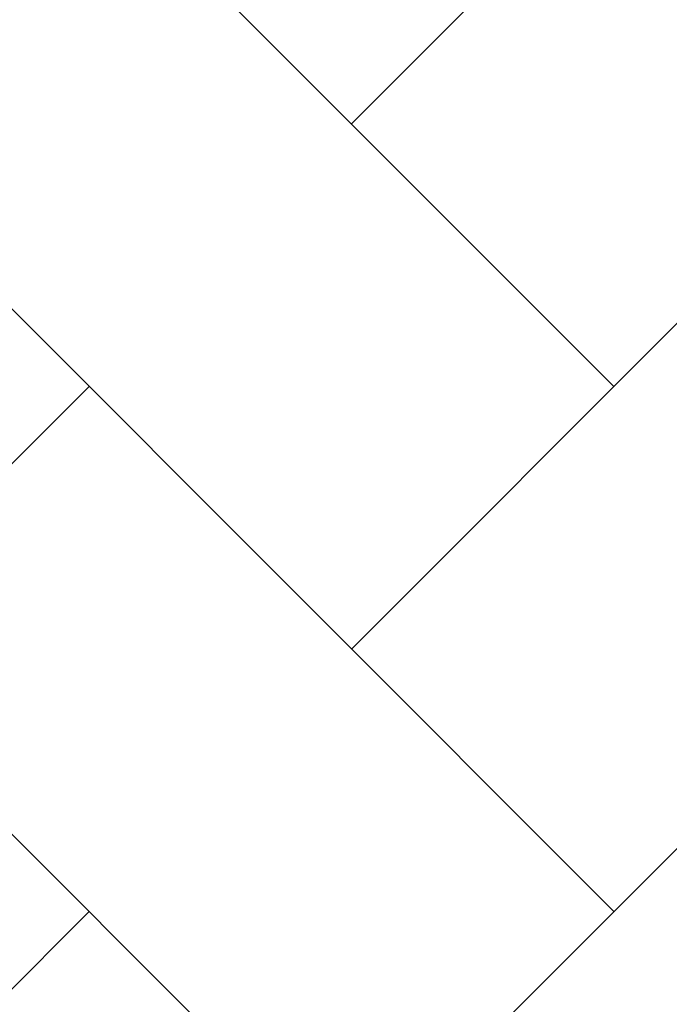
# Model space of a CAD drawing. Units: inches. Extents: x 3590 to 5167, y 65 to 1917.
# Tile 55 of 100: x 4968 to 5003, y 1504 to 1558. Entities that reach past the tile are written whole.
import ezdxf

# ---------------------------------------------------------------- set-up
doc = ezdxf.new("R2010")
doc.units = ezdxf.units.IN
doc.layers.add('A-FLOR-PATT', color=8, linetype='Continuous', lineweight=13)

msp = doc.modelspace()

# ---------------------------------------------------------------- hatches: boundary and pattern name
at = {"layer": 'A-FLOR-PATT', "transparency": 33554687}
h = msp.add_hatch(dxfattribs=at)
h.set_pattern_fill('AR-HBONE', color=256, scale=0.2)
h.set_pattern_definition([(45, (-588.972, 0), (0, 28.73682), [60.96, -20.32]), (135, (-574.604, 14.368), (3e-15, 28.73682), [60.96, -20.32])])
h.paths.add_polyline_path([(5071.274, 1796.999), (4933.274, 1796.999), (4933.274, 1753.999), (4962.774, 1753.999, -0.414214), (4928.774, 1719.999), (4933.274, 1718.999), (4933.274, 1334.999), (5071.274, 1334.999)])
h.paths.add_polyline_path([(4951.78, 1521.077), (4951.715, 1521.04), (4951.563, 1520.895)], flags=16)
h.paths.add_polyline_path([(4952.267, 1521.376), (4952.198, 1521.371), (4952.198, 1521.356)], flags=0)
h.paths.add_polyline_path([(4967.051, 1529.728), (4965.231, 1528.694), (4963.411, 1527.714), (4961.756, 1526.851), (4963.589, 1527.449), (4964.036, 1527.478), (4962.975, 1527.249), (4961.76, 1526.852), (4959.792, 1525.834), (4958.005, 1524.895), (4956.24, 1523.93), (4954.504, 1522.919), (4954.129, 1522.682), (4953.361, 1521.997), (4953.366, 1521.998), (4953.605, 1522.064), (4955.106, 1522.761), (4956.921, 1523.434), (4958.678, 1523.915), (4960.358, 1524.2), (4961.945, 1524.286), (4964.171, 1524.108), (4965.958, 1523.309), (4963.863, 1522.976), (4965.187, 1522.499), (4963.366, 1522.497), (4961.545, 1522.487), (4959.764, 1522.461), (4958.304, 1522.419), (4957.974, 1522.388), (4956.307, 1522.232), (4954.718, 1522.071), (4953.251, 1521.899), (4953.525, 1521.623), (4954.331, 1521.379), (4956.243, 1521.23), (4958.039, 1520.93), (4959.684, 1520.483), (4961.16, 1519.896), (4963.107, 1518.8), (4964.393, 1517.325), (4962.973, 1517.726), (4964.558, 1516.661), (4965.407, 1515.708), (4963.507, 1516.322), (4961.68, 1517.005), (4959.935, 1517.745), (4958.282, 1518.528), (4956.732, 1519.343), (4955.295, 1520.175), (4954.672, 1520.572), (4954.513, 1520.627), (4955.658, 1519.318), (4956.703, 1517.982), (4957.644, 1516.647), (4958.485, 1515.334), (4959.55, 1513.524), (4960.438, 1511.769), (4958.841, 1513.62), (4957.452, 1515.325), (4955.819, 1517.459), (4956.665, 1515.448), (4957.111, 1513.923), (4957.447, 1511.714), (4957.076, 1509.793), (4956.538, 1511.11), (4955.992, 1512.569), (4955.444, 1514.125), (4954.898, 1515.735), (4954.357, 1517.356), (4953.824, 1518.943), (4953.305, 1520.452), (4953.065, 1521.116), (4952.971, 1521.146), (4952.949, 1521.086), (4952.73, 1520.199), (4953.37, 1518.024), (4953.757, 1516.373), (4954.051, 1514.765), (4954.264, 1513.221), (4954.471, 1511.131), (4954.497, 1510.402), (4954.409, 1511.76), (4954.264, 1513.221), (4954.051, 1514.765), (4953.757, 1516.373), (4953.37, 1518.024), (4952.877, 1519.698), (4952.716, 1520.141), (4952.533, 1519.059), (4952.374, 1517.789), (4952.219, 1516.312), (4952.046, 1514.6), (4951.833, 1512.626), (4951.557, 1510.363), (4951.203, 1512.168), (4950.852, 1514.339), (4950.985, 1516.376), (4951.66, 1518.286), (4952.593, 1520.481), (4952.357, 1521.13), (4951.855, 1520.328), (4950.839, 1518.908), (4949.777, 1517.587), (4948.916, 1516.617), (4948.111, 1515.256), (4947.089, 1513.554), (4945.889, 1511.615), (4946.326, 1513.402), (4946.562, 1514.249), (4945.528, 1513.327), (4944.581, 1512.531), (4946.018, 1514.508), (4947.204, 1516.048), (4947.893, 1517.313), (4949.307, 1518.764), (4950.414, 1519.767), (4950.451, 1519.806), (4952.267, 1521.376), (4951.645, 1521.493), (4950.404, 1521.18), (4948.044, 1520.359), (4946.119, 1519.452), (4944.572, 1518.475), (4943.35, 1517.443), (4941.997, 1515.92), (4941.661, 1515.275), (4942.813, 1516.99), (4944.572, 1518.475), (4946.119, 1519.452), (4948.044, 1520.359), (4950.404, 1521.18), (4951.645, 1521.493), (4949.647, 1521.868), (4948.6, 1521.756), (4947.126, 1521.57), (4945.42, 1521.348), (4943.45, 1521.105), (4941.183, 1520.856), (4942.86, 1521.613), (4943.873, 1522.03), (4942.952, 1521.909), (4941.41, 1521.485), (4939.543, 1520.67), (4938.968, 1520.226), (4940.733, 1521.299), (4942.952, 1521.909), (4943.702, 1522.008), (4945.894, 1522.7), (4947.565, 1522.714), (4948.921, 1522.566), (4951.131, 1522.183), (4950.971, 1522.297), (4948.129, 1523.006), (4946.035, 1523.707), (4944.232, 1524.521), (4942.707, 1525.461), (4941.444, 1526.537), (4940.43, 1527.761), (4939.649, 1529.143), (4941.421, 1528.122), (4943.147, 1527.132), (4944.841, 1526.175), (4946.514, 1525.25), (4948.179, 1524.359), (4948.365, 1524.263), (4946.475, 1526.045), (4945.181, 1527.54), (4944.19, 1529.033), (4943.496, 1530.54), (4943.278, 1531.36), (4942.498, 1531.919), (4943.114, 1531.762), (4942.959, 1533.659), (4944.14, 1531.989), (4944.612, 1531.323), (4946.202, 1530.463), (4947.486, 1529.509), (4948.79, 1528.226), (4950.368, 1526.237), (4949.485, 1528.155), (4948.851, 1530.123), (4948.491, 1532.041), (4948.381, 1533.918), (4948.501, 1535.76), (4948.827, 1537.573), (4949.418, 1535.565), (4949.957, 1533.569), (4950.464, 1531.586), (4950.961, 1529.617), (4951.391, 1527.954), (4951.724, 1530.687), (4952.201, 1532.58), (4952.889, 1534.33), (4953.77, 1535.951), (4954.827, 1537.46), (4954.521, 1535.39), (4954.273, 1533.937), (4955.58, 1535.663), (4956.748, 1536.739), (4956.159, 1534.78), (4955.589, 1532.873), (4955.043, 1531.006), (4954.525, 1529.166), (4954.038, 1527.341), (4953.638, 1525.733), (4953.611, 1525.586), (4953.398, 1524.166), (4953.382, 1524.009), (4954.07, 1525.476), (4954.912, 1527.022), (4956.136, 1528.894), (4957.847, 1530.577), (4959.376, 1531.54), (4958.256, 1530.104), (4957.143, 1528.663), (4956.066, 1527.243), (4955.056, 1525.871), (4954.141, 1524.571), (4953.352, 1523.372), (4953.311, 1523.303), (4953.273, 1522.925), (4953.261, 1522.382), (4954.103, 1523.373), (4954.63, 1524.284), (4955.961, 1526.358), (4957.23, 1528.13), (4958.421, 1529.609), (4960.037, 1531.368), (4961.374, 1532.375), (4962.101, 1532.77), (4961.07, 1531.061), (4959.987, 1529.438), (4958.869, 1527.908), (4958.15, 1527.007), (4959.803, 1528.003), (4961.589, 1528.793), (4963.391, 1529.328), (4965.211, 1529.632)], flags=16)
h.paths.add_polyline_path([(4962.944, 1523.182), (4961.107, 1523.422), (4960.392, 1523.362), (4962.35, 1523.331)], flags=0)
h.paths.add_polyline_path([(5049.541, 1584.551), (5049.476, 1584.515), (5049.325, 1584.37)], flags=16)
h.paths.add_polyline_path([(5050.028, 1584.851), (5049.959, 1584.845), (5049.959, 1584.83)], flags=0)
h.paths.add_polyline_path([(5042.333, 1581.949), (5043.88, 1582.926), (5045.806, 1583.833), (5048.165, 1584.654), (5049.406, 1584.967), (5047.408, 1585.342), (5046.361, 1585.231), (5044.888, 1585.044), (5043.181, 1584.822), (5041.211, 1584.579), (5038.944, 1584.33), (5040.622, 1585.087), (5041.634, 1585.504), (5040.713, 1585.383), (5039.171, 1584.959), (5037.304, 1584.144), (5036.729, 1583.7), (5038.494, 1584.773), (5040.713, 1585.383), (5041.463, 1585.482), (5043.655, 1586.174), (5045.326, 1586.188), (5046.682, 1586.04), (5048.893, 1585.657), (5048.732, 1585.771), (5045.891, 1586.48), (5043.796, 1587.181), (5041.994, 1587.996), (5040.468, 1588.935), (5039.205, 1590.011), (5038.191, 1591.235), (5037.41, 1592.617), (5039.182, 1591.596), (5040.909, 1590.607), (5042.602, 1589.649), (5044.275, 1588.724), (5045.94, 1587.833), (5046.126, 1587.738), (5044.237, 1589.519), (5042.942, 1591.015), (5041.952, 1592.508), (5041.257, 1594.014), (5041.039, 1594.834), (5040.26, 1595.393), (5040.875, 1595.237), (5040.721, 1597.133), (5041.901, 1595.463), (5042.373, 1594.798), (5043.963, 1593.938), (5045.247, 1592.983), (5046.552, 1591.701), (5048.129, 1589.712), (5047.247, 1591.63), (5046.613, 1593.597), (5046.252, 1595.515), (5046.142, 1597.392), (5046.262, 1599.234), (5046.588, 1601.047), (5047.179, 1599.039), (5047.718, 1597.043), (5048.225, 1595.06), (5048.722, 1593.091), (5049.152, 1591.429), (5049.485, 1594.161), (5049.962, 1596.054), (5050.65, 1597.804), (5051.532, 1599.425), (5052.589, 1600.934), (5052.283, 1598.864), (5052.034, 1597.411), (5053.341, 1599.137), (5054.509, 1600.213), (5053.92, 1598.254), (5053.35, 1596.348), (5052.805, 1594.48), (5052.286, 1592.64), (5051.799, 1590.815), (5051.4, 1589.207), (5051.373, 1589.06), (5051.159, 1587.64), (5051.143, 1587.483), (5051.831, 1588.95), (5052.673, 1590.496), (5053.898, 1592.368), (5055.608, 1594.051), (5057.137, 1595.014), (5056.017, 1593.578), (5054.904, 1592.137), (5053.828, 1590.717), (5052.817, 1589.345), (5051.902, 1588.046), (5051.113, 1586.846), (5051.072, 1586.777), (5051.034, 1586.399), (5051.022, 1585.856), (5051.864, 1586.847), (5052.391, 1587.758), (5053.723, 1589.832), (5054.991, 1591.604), (5056.182, 1593.083), (5057.798, 1594.842), (5059.135, 1595.849), (5059.863, 1596.244), (5058.831, 1594.535), (5057.749, 1592.912), (5056.63, 1591.382), (5055.912, 1590.482), (5057.564, 1591.477), (5059.35, 1592.267), (5061.152, 1592.802), (5062.972, 1593.106), (5064.812, 1593.203), (5062.992, 1592.169), (5061.172, 1591.188), (5059.518, 1590.325), (5061.35, 1590.924), (5061.797, 1590.952), (5060.737, 1590.723), (5059.521, 1590.326), (5057.553, 1589.308), (5055.766, 1588.369), (5054.002, 1587.404), (5052.265, 1586.393), (5051.891, 1586.156), (5051.122, 1585.471), (5051.127, 1585.472), (5051.366, 1585.538), (5052.867, 1586.235), (5054.682, 1586.908), (5056.439, 1587.389), (5058.12, 1587.675), (5059.706, 1587.76), (5061.933, 1587.583), (5063.719, 1586.783), (5061.624, 1586.45), (5062.949, 1585.973), (5061.127, 1585.971), (5059.307, 1585.961), (5057.525, 1585.935), (5056.065, 1585.893), (5055.735, 1585.862), (5054.068, 1585.707), (5052.479, 1585.546), (5051.012, 1585.373), (5051.286, 1585.097), (5052.092, 1584.853), (5054.004, 1584.704), (5055.8, 1584.404), (5057.446, 1583.958), (5058.921, 1583.37), (5060.868, 1582.274), (5062.154, 1580.799), (5060.734, 1581.2), (5062.32, 1580.135), (5063.168, 1579.182), (5061.269, 1579.796), (5059.441, 1580.479), (5057.696, 1581.219), (5056.043, 1582.003), (5054.493, 1582.817), (5053.057, 1583.649), (5052.433, 1584.047), (5052.274, 1584.101), (5053.42, 1582.793), (5054.464, 1581.457), (5055.405, 1580.121), (5056.247, 1578.809), (5057.311, 1576.998), (5058.199, 1575.244), (5056.602, 1577.094), (5055.213, 1578.799), (5053.58, 1580.933), (5054.427, 1578.922), (5054.872, 1577.397), (5055.208, 1575.189), (5054.838, 1573.267), (5054.299, 1574.584), (5053.754, 1576.043), (5053.206, 1577.599), (5052.659, 1579.209), (5052.118, 1580.83), (5051.585, 1582.417), (5051.066, 1583.927), (5050.826, 1584.59), (5050.733, 1584.62), (5050.711, 1584.561), (5050.491, 1583.673), (5051.131, 1581.498), (5051.518, 1579.847), (5051.813, 1578.24), (5052.026, 1576.695), (5052.233, 1574.605), (5052.258, 1573.876), (5052.17, 1575.234), (5052.026, 1576.695), (5051.813, 1578.24), (5051.518, 1579.847), (5051.131, 1581.498), (5050.638, 1583.172), (5050.477, 1583.615), (5050.294, 1582.533), (5050.136, 1581.263), (5049.981, 1579.786), (5049.807, 1578.074), (5049.594, 1576.1), (5049.318, 1573.837), (5048.965, 1575.642), (5048.613, 1577.813), (5048.747, 1579.85), (5049.421, 1581.76), (5050.354, 1583.955), (5050.118, 1584.604), (5049.616, 1583.802), (5048.6, 1582.382), (5047.538, 1581.061), (5046.677, 1580.091), (5045.872, 1578.73), (5044.85, 1577.028), (5043.651, 1575.089), (5044.087, 1576.877), (5044.324, 1577.723), (5043.289, 1576.801), (5042.342, 1576.005), (5043.779, 1577.982), (5044.966, 1579.522), (5045.655, 1580.787), (5047.068, 1582.239), (5048.175, 1583.241), (5048.213, 1583.28), (5050.028, 1584.851), (5049.406, 1584.967), (5048.165, 1584.654), (5045.806, 1583.833), (5043.88, 1582.926), (5042.333, 1581.949), (5041.111, 1580.917), (5039.758, 1579.394), (5039.423, 1578.749), (5040.575, 1580.464)], flags=16)
h.paths.add_polyline_path([(4954.799, 1533.12), (4954.262, 1532.079), (4953.831, 1530.935), (4953.505, 1529.636), (4953.283, 1528.133), (4953.167, 1526.376), (4953.156, 1524.315), (4953.277, 1521.236), (4952.802, 1521.842), (4951.557, 1521.998), (4950.976, 1521.961), (4952.661, 1521.941), (4952.802, 1521.842), (4953.152, 1523.593), (4953.167, 1526.376), (4953.283, 1528.133), (4953.609, 1530.346), (4954.456, 1532.592)], flags=0)
h.paths.add_polyline_path([(5050.563, 1585.316), (5049.318, 1585.472), (5048.737, 1585.435), (5050.422, 1585.415), (5050.563, 1585.316), (5050.914, 1587.067), (5050.928, 1589.851), (5051.045, 1591.607), (5051.371, 1593.82), (5052.217, 1596.066), (5052.56, 1596.594), (5052.024, 1595.554), (5051.592, 1594.409), (5051.266, 1593.11), (5051.045, 1591.607), (5050.928, 1589.851), (5050.918, 1587.789), (5051.038, 1584.71)], flags=0)
h.paths.add_polyline_path([(5058.153, 1586.836), (5060.111, 1586.805), (5060.705, 1586.656), (5058.868, 1586.896)], flags=0)
h.paths.add_polyline_path([(5049.541, 1430.936), (5049.476, 1430.9), (5049.325, 1430.755)], flags=16)
h.paths.add_polyline_path([(5050.028, 1431.236), (5049.959, 1431.231), (5049.959, 1431.215)], flags=0)
h.paths.add_polyline_path([(5046.588, 1447.432), (5047.179, 1445.425), (5047.718, 1443.429), (5048.225, 1441.446), (5048.722, 1439.476), (5049.152, 1437.814), (5049.485, 1440.546), (5049.962, 1442.439), (5050.65, 1444.189), (5051.532, 1445.811), (5052.589, 1447.319), (5052.283, 1445.249), (5052.034, 1443.796), (5053.341, 1445.522), (5054.509, 1446.598), (5053.92, 1444.64), (5053.35, 1442.733), (5052.805, 1440.865), (5052.286, 1439.025), (5051.799, 1437.201), (5051.4, 1435.592), (5051.373, 1435.445), (5051.159, 1434.025), (5051.143, 1433.868), (5051.831, 1435.335), (5052.673, 1436.881), (5053.898, 1438.753), (5055.608, 1440.436), (5057.137, 1441.4), (5056.017, 1439.963), (5054.904, 1438.522), (5053.828, 1437.102), (5052.817, 1435.73), (5051.902, 1434.431), (5051.113, 1433.231), (5051.072, 1433.162), (5051.034, 1432.784), (5051.022, 1432.242), (5051.864, 1433.232), (5052.391, 1434.143), (5053.723, 1436.217), (5054.991, 1437.989), (5056.182, 1439.468), (5057.798, 1441.227), (5059.135, 1442.235), (5059.863, 1442.629), (5058.831, 1440.921), (5057.749, 1439.298), (5056.63, 1437.767), (5055.912, 1436.867), (5057.564, 1437.863), (5059.35, 1438.652), (5061.152, 1439.187), (5062.972, 1439.491), (5064.812, 1439.588), (5062.992, 1438.554), (5061.172, 1437.573), (5059.518, 1436.71), (5061.35, 1437.309), (5061.797, 1437.337), (5060.737, 1437.108), (5059.521, 1436.711), (5057.553, 1435.693), (5055.766, 1434.754), (5054.002, 1433.789), (5052.265, 1432.778), (5051.891, 1432.541), (5051.122, 1431.856), (5051.127, 1431.857), (5051.366, 1431.923), (5052.867, 1432.62), (5054.682, 1433.293), (5056.439, 1433.775), (5058.12, 1434.06), (5059.706, 1434.145), (5061.933, 1433.968), (5063.719, 1433.168), (5061.624, 1432.835), (5062.949, 1432.358), (5061.127, 1432.357), (5059.307, 1432.346), (5057.525, 1432.32), (5056.065, 1432.278), (5055.735, 1432.248), (5054.068, 1432.092), (5052.479, 1431.931), (5051.012, 1431.759), (5051.286, 1431.482), (5052.092, 1431.238), (5054.004, 1431.089), (5055.8, 1430.789), (5057.446, 1430.343), (5058.921, 1429.755), (5060.868, 1428.66), (5062.154, 1427.185), (5060.734, 1427.585), (5062.32, 1426.52), (5063.168, 1425.567), (5061.269, 1426.181), (5059.441, 1426.865), (5057.696, 1427.604), (5056.043, 1428.388), (5054.493, 1429.202), (5053.057, 1430.034), (5052.433, 1430.432), (5052.274, 1430.487), (5053.42, 1429.178), (5054.464, 1427.842), (5055.405, 1426.506), (5056.247, 1425.194), (5057.311, 1423.383), (5058.199, 1421.629), (5056.602, 1423.479), (5055.213, 1425.184), (5053.58, 1427.318), (5054.427, 1425.307), (5054.872, 1423.782), (5055.208, 1421.574), (5054.838, 1419.652), (5054.299, 1420.97), (5053.754, 1422.428), (5053.206, 1423.984), (5052.659, 1425.595), (5052.118, 1427.215), (5051.585, 1428.802), (5051.066, 1430.312), (5050.826, 1430.975), (5050.733, 1431.005), (5050.711, 1430.946), (5050.491, 1430.058), (5051.131, 1427.883), (5051.518, 1426.232), (5051.813, 1424.625), (5052.026, 1423.081), (5052.233, 1420.991), (5052.258, 1420.261), (5052.17, 1421.619), (5052.026, 1423.081), (5051.813, 1424.625), (5051.518, 1426.232), (5051.131, 1427.883), (5050.638, 1429.558), (5050.477, 1430.001), (5050.294, 1428.918), (5050.136, 1427.648), (5049.981, 1426.171), (5049.807, 1424.459), (5049.594, 1422.485), (5049.318, 1420.222), (5048.965, 1422.028), (5048.613, 1424.199), (5048.747, 1426.235), (5049.421, 1428.146), (5050.354, 1430.34), (5050.118, 1430.989), (5049.616, 1430.187), (5048.6, 1428.768), (5047.538, 1427.446), (5046.677, 1426.477), (5045.872, 1425.116), (5044.85, 1423.413), (5043.651, 1421.474), (5044.087, 1423.262), (5044.324, 1424.109), (5043.289, 1423.186), (5042.342, 1422.391), (5043.779, 1424.368), (5044.966, 1425.907), (5045.655, 1427.173), (5047.068, 1428.624), (5048.175, 1429.627), (5048.213, 1429.666), (5050.028, 1431.236), (5049.406, 1431.353), (5048.165, 1431.039), (5045.806, 1430.218), (5043.88, 1429.311), (5042.333, 1428.334), (5041.111, 1427.302), (5039.758, 1425.779), (5039.423, 1425.134), (5040.575, 1426.849), (5042.333, 1428.334), (5043.88, 1429.311), (5045.806, 1430.218), (5048.165, 1431.039), (5049.406, 1431.353), (5047.408, 1431.727), (5046.361, 1431.616), (5044.888, 1431.429), (5043.181, 1431.207), (5041.211, 1430.964), (5038.944, 1430.715), (5040.622, 1431.472), (5041.634, 1431.89), (5040.713, 1431.769), (5039.171, 1431.345), (5037.304, 1430.53), (5036.729, 1430.085), (5038.494, 1431.158), (5040.713, 1431.769), (5041.463, 1431.867), (5043.655, 1432.559), (5045.326, 1432.573), (5046.682, 1432.425), (5048.893, 1432.042), (5048.732, 1432.156), (5045.891, 1432.865), (5043.796, 1433.566), (5041.994, 1434.381), (5040.468, 1435.321), (5039.205, 1436.396), (5038.191, 1437.62), (5037.41, 1439.002), (5039.182, 1437.982), (5040.909, 1436.992), (5042.602, 1436.034), (5044.275, 1435.109), (5045.94, 1434.218), (5046.126, 1434.123), (5044.237, 1435.904), (5042.942, 1437.4), (5041.952, 1438.893), (5041.257, 1440.399), (5041.039, 1441.219), (5040.26, 1441.778), (5040.875, 1441.622), (5040.721, 1443.518), (5041.901, 1441.848), (5042.373, 1441.183), (5043.963, 1440.323), (5045.247, 1439.369), (5046.552, 1438.086), (5048.129, 1436.097), (5047.247, 1438.015), (5046.613, 1439.982), (5046.252, 1441.901), (5046.142, 1443.778), (5046.262, 1445.619)], flags=16)
h.paths.add_polyline_path([(5052.382, 1444.255), (5051.623, 1442.78), (5052.024, 1441.939), (5052.56, 1442.98)], flags=0)
h.paths.add_polyline_path([(5050.563, 1431.701), (5049.318, 1431.857), (5048.737, 1431.821), (5050.422, 1431.8)], flags=0)
h.paths.add_polyline_path([(5058.153, 1433.221), (5060.111, 1433.19), (5060.705, 1433.041), (5058.868, 1433.281)], flags=0)
h.paths.add_polyline_path([(5049.541, 1352.285), (5049.476, 1352.249), (5049.325, 1352.104)], flags=16)
h.paths.add_polyline_path([(5050.028, 1352.585), (5049.959, 1352.58), (5049.959, 1352.564)], flags=0)
h.paths.add_polyline_path([(5046.588, 1368.781), (5047.179, 1366.774), (5047.718, 1364.778), (5048.225, 1362.795), (5048.722, 1360.825), (5049.152, 1359.163), (5049.485, 1361.896), (5049.962, 1363.789), (5050.65, 1365.538), (5051.532, 1367.16), (5052.589, 1368.669), (5052.283, 1366.598), (5052.034, 1365.145), (5053.341, 1366.871), (5054.509, 1367.947), (5053.92, 1365.989), (5053.35, 1364.082), (5052.805, 1362.214), (5052.286, 1360.374), (5051.799, 1358.55), (5051.4, 1356.942), (5051.373, 1356.794), (5051.159, 1355.374), (5051.143, 1355.218), (5051.831, 1356.684), (5052.673, 1358.23), (5053.898, 1360.102), (5055.608, 1361.786), (5057.137, 1362.749), (5056.017, 1361.313), (5054.904, 1359.872), (5053.828, 1358.452), (5052.817, 1357.079), (5051.902, 1355.78), (5051.113, 1354.581), (5051.072, 1354.512), (5051.034, 1354.133), (5051.022, 1353.591), (5051.864, 1354.581), (5052.391, 1355.492), (5053.723, 1357.566), (5054.991, 1359.338), (5056.182, 1360.817), (5057.798, 1362.577), (5059.135, 1363.584), (5059.863, 1363.979), (5058.831, 1362.27), (5057.749, 1360.647), (5056.63, 1359.117), (5055.912, 1358.216), (5057.564, 1359.212), (5059.35, 1360.001), (5061.152, 1360.536), (5062.972, 1360.841), (5064.812, 1360.937), (5062.992, 1359.903), (5061.172, 1358.923), (5059.518, 1358.059), (5061.35, 1358.658), (5061.797, 1358.687), (5060.737, 1358.458), (5059.521, 1358.061), (5057.553, 1357.043), (5055.766, 1356.103), (5054.002, 1355.138), (5052.265, 1354.127), (5051.891, 1353.89), (5051.122, 1353.206), (5051.127, 1353.206), (5051.366, 1353.272), (5052.867, 1353.969), (5054.682, 1354.643), (5056.439, 1355.124), (5058.12, 1355.409), (5059.706, 1355.495), (5061.933, 1355.317), (5063.719, 1354.518), (5061.624, 1354.184), (5062.949, 1353.708), (5061.127, 1353.706), (5059.307, 1353.695), (5057.525, 1353.669), (5056.065, 1353.627), (5055.735, 1353.597), (5054.068, 1353.441), (5052.479, 1353.28), (5051.012, 1353.108), (5051.286, 1352.831), (5052.092, 1352.587), (5054.004, 1352.439), (5055.8, 1352.138), (5057.446, 1351.692), (5058.921, 1351.104), (5060.868, 1350.009), (5062.154, 1348.534), (5060.734, 1348.935), (5062.32, 1347.869), (5063.168, 1346.916), (5061.269, 1347.53), (5059.441, 1348.214), (5057.696, 1348.954), (5056.043, 1349.737), (5054.493, 1350.551), (5053.057, 1351.383), (5052.433, 1351.781), (5052.274, 1351.836), (5053.42, 1350.527), (5054.464, 1349.191), (5055.405, 1347.855), (5056.247, 1346.543), (5057.311, 1344.733), (5058.199, 1342.978), (5056.602, 1344.828), (5055.213, 1346.534), (5053.58, 1348.667), (5054.427, 1346.656), (5054.872, 1345.132), (5055.208, 1342.923), (5054.838, 1341.002), (5054.299, 1342.319), (5053.754, 1343.778), (5053.206, 1345.334), (5052.659, 1346.944), (5052.118, 1348.564), (5051.585, 1350.151), (5051.066, 1351.661), (5050.826, 1352.324), (5050.733, 1352.355), (5050.711, 1352.295), (5050.491, 1351.408), (5051.131, 1349.232), (5051.518, 1347.581), (5051.813, 1345.974), (5052.026, 1344.43), (5052.233, 1342.34), (5052.258, 1341.61), (5052.17, 1342.969), (5052.026, 1344.43), (5051.813, 1345.974), (5051.518, 1347.581), (5051.131, 1349.232), (5050.638, 1350.907), (5050.477, 1351.35), (5050.294, 1350.267), (5050.136, 1348.997), (5049.981, 1347.52), (5049.807, 1345.809), (5049.594, 1343.835), (5049.318, 1341.571), (5048.965, 1343.377), (5048.613, 1345.548), (5048.747, 1347.585), (5049.421, 1349.495), (5050.354, 1351.689), (5050.118, 1352.339), (5049.616, 1351.536), (5048.6, 1350.117), (5047.538, 1348.795), (5046.677, 1347.826), (5045.872, 1346.465), (5044.85, 1344.763), (5043.651, 1342.824), (5044.087, 1344.611), (5044.324, 1345.458), (5043.289, 1344.535), (5042.342, 1343.74), (5043.779, 1345.717), (5044.966, 1347.256), (5045.655, 1348.522), (5047.068, 1349.973), (5048.175, 1350.976), (5048.213, 1351.015), (5050.028, 1352.585), (5049.406, 1352.702), (5048.165, 1352.388), (5045.806, 1351.567), (5043.88, 1350.661), (5042.333, 1349.683), (5041.111, 1348.651), (5039.758, 1347.128), (5039.423, 1346.483), (5040.575, 1348.198), (5042.333, 1349.683), (5043.88, 1350.661), (5045.806, 1351.567), (5048.165, 1352.388), (5049.406, 1352.702), (5047.408, 1353.076), (5046.361, 1352.965), (5044.888, 1352.779), (5043.181, 1352.556), (5041.211, 1352.313), (5038.944, 1352.065), (5040.622, 1352.821), (5041.634, 1353.239), (5040.713, 1353.118), (5039.171, 1352.694), (5037.304, 1351.879), (5036.729, 1351.434), (5038.494, 1352.508), (5040.713, 1353.118), (5041.463, 1353.216), (5043.655, 1353.909), (5045.326, 1353.923), (5046.682, 1353.774), (5048.893, 1353.391), (5048.732, 1353.506), (5045.891, 1354.214), (5043.796, 1354.915), (5041.994, 1355.73), (5040.468, 1356.67), (5039.205, 1357.746), (5038.191, 1358.969), (5037.41, 1360.352), (5039.182, 1359.331), (5040.909, 1358.341), (5042.602, 1357.383), (5044.275, 1356.458), (5045.94, 1355.567), (5046.126, 1355.472), (5044.237, 1357.253), (5042.942, 1358.749), (5041.952, 1360.242), (5041.257, 1361.748), (5041.039, 1362.568), (5040.26, 1363.128), (5040.875, 1362.971), (5040.721, 1364.867), (5041.901, 1363.197), (5042.373, 1362.532), (5043.963, 1361.672), (5045.247, 1360.718), (5046.552, 1359.435), (5048.129, 1357.446), (5047.247, 1359.364), (5046.613, 1361.331), (5046.252, 1363.25), (5046.142, 1365.127), (5046.262, 1366.969)], flags=16)
h.paths.add_polyline_path([(5052.382, 1365.604), (5051.623, 1364.129), (5052.024, 1363.288), (5052.56, 1364.329)], flags=0)
h.paths.add_polyline_path([(4951.78, 1698.041), (4951.715, 1698.005), (4951.563, 1697.859)], flags=16)
h.paths.add_polyline_path([(4952.267, 1698.341), (4952.198, 1698.335), (4952.198, 1698.32)], flags=0)
h.paths.add_polyline_path([(4957.076, 1686.757), (4956.538, 1688.074), (4955.992, 1689.533), (4955.444, 1691.089), (4954.898, 1692.699), (4954.357, 1694.32), (4953.824, 1695.907), (4953.305, 1697.417), (4953.065, 1698.08), (4952.971, 1698.11), (4952.949, 1698.051), (4952.73, 1697.163), (4953.37, 1694.988), (4953.757, 1693.337), (4954.051, 1691.729), (4954.264, 1690.185), (4954.471, 1688.095), (4954.497, 1687.366), (4954.409, 1688.724), (4954.264, 1690.185), (4954.051, 1691.729), (4953.757, 1693.337), (4953.37, 1694.988), (4952.877, 1696.662), (4952.716, 1697.105), (4952.533, 1696.023), (4952.374, 1694.753), (4952.219, 1693.276), (4952.046, 1691.564), (4951.833, 1689.59), (4951.557, 1687.327), (4951.203, 1689.132), (4950.852, 1691.303), (4950.985, 1693.34), (4951.66, 1695.25), (4952.593, 1697.445), (4952.357, 1698.094), (4951.855, 1697.292), (4950.839, 1695.872), (4949.777, 1694.551), (4948.916, 1693.581), (4948.111, 1692.22), (4947.089, 1690.518), (4945.889, 1688.579), (4946.326, 1690.366), (4946.562, 1691.213), (4945.528, 1690.291), (4944.581, 1689.495), (4946.018, 1691.472), (4947.204, 1693.012), (4947.893, 1694.277), (4949.307, 1695.729), (4950.414, 1696.731), (4950.451, 1696.77), (4952.267, 1698.341), (4951.645, 1698.457), (4950.404, 1698.144), (4948.044, 1697.323), (4946.119, 1696.416), (4944.572, 1695.439), (4943.35, 1694.407), (4941.997, 1692.884), (4941.661, 1692.239), (4942.813, 1693.954), (4944.572, 1695.439), (4946.119, 1696.416), (4948.044, 1697.323), (4950.404, 1698.144), (4951.645, 1698.457), (4949.647, 1698.832), (4948.6, 1698.72), (4947.126, 1698.534), (4945.42, 1698.312), (4943.45, 1698.069), (4941.183, 1697.82), (4942.86, 1698.577), (4943.873, 1698.994), (4942.952, 1698.873), (4941.41, 1698.449), (4939.543, 1697.634), (4938.968, 1697.19), (4940.733, 1698.263), (4942.952, 1698.873), (4943.702, 1698.972), (4945.894, 1699.664), (4947.565, 1699.678), (4948.921, 1699.53), (4951.131, 1699.147), (4950.971, 1699.261), (4948.129, 1699.97), (4946.035, 1700.671), (4944.232, 1701.486), (4942.707, 1702.425), (4941.444, 1703.501), (4940.43, 1704.725), (4939.649, 1706.107), (4941.421, 1705.086), (4943.147, 1704.097), (4944.841, 1703.139), (4946.514, 1702.214), (4948.179, 1701.323), (4948.365, 1701.227), (4946.475, 1703.009), (4945.181, 1704.505), (4944.19, 1705.997), (4943.496, 1707.504), (4943.278, 1708.324), (4942.498, 1708.883), (4943.114, 1708.727), (4942.959, 1710.623), (4944.14, 1708.953), (4944.612, 1708.287), (4946.202, 1707.428), (4947.486, 1706.473), (4948.79, 1705.191), (4950.368, 1703.202), (4949.485, 1705.12), (4948.851, 1707.087), (4948.491, 1709.005), (4948.381, 1710.882), (4948.501, 1712.724), (4948.827, 1714.537), (4949.418, 1712.529), (4949.957, 1710.533), (4950.464, 1708.55), (4950.961, 1706.581), (4951.391, 1704.919), (4951.724, 1707.651), (4952.201, 1709.544), (4952.889, 1711.294), (4953.77, 1712.915), (4954.827, 1714.424), (4954.521, 1712.354), (4954.273, 1710.901), (4955.58, 1712.627), (4956.748, 1713.703), (4956.159, 1711.744), (4955.589, 1709.837), (4955.043, 1707.97), (4954.525, 1706.13), (4954.038, 1704.305), (4953.638, 1702.697), (4953.611, 1702.55), (4953.398, 1701.13), (4953.382, 1700.973), (4954.07, 1702.44), (4954.912, 1703.986), (4956.136, 1705.858), (4957.847, 1707.541), (4959.376, 1708.504), (4958.256, 1707.068), (4957.143, 1705.627), (4956.066, 1704.207), (4955.056, 1702.835), (4954.141, 1701.536), (4953.352, 1700.336), (4953.311, 1700.267), (4953.273, 1699.889), (4953.261, 1699.346), (4954.103, 1700.337), (4954.63, 1701.248), (4955.961, 1703.322), (4957.23, 1705.094), (4958.421, 1706.573), (4960.037, 1708.332), (4961.374, 1709.339), (4962.101, 1709.734), (4961.07, 1708.025), (4959.987, 1706.402), (4958.869, 1704.872), (4958.15, 1703.972), (4959.803, 1704.967), (4961.589, 1705.757), (4963.391, 1706.292), (4965.211, 1706.596), (4967.051, 1706.692), (4965.231, 1705.659), (4963.411, 1704.678), (4961.756, 1703.815), (4963.589, 1704.413), (4964.036, 1704.442), (4962.975, 1704.213), (4961.76, 1703.816), (4959.792, 1702.798), (4958.005, 1701.859), (4956.24, 1700.894), (4954.504, 1699.883), (4954.129, 1699.646), (4953.361, 1698.961), (4953.366, 1698.962), (4953.605, 1699.028), (4955.106, 1699.725), (4956.921, 1700.398), (4958.678, 1700.879), (4960.358, 1701.164), (4961.945, 1701.25), (4964.171, 1701.073), (4965.958, 1700.273), (4963.863, 1699.94), (4965.187, 1699.463), (4963.366, 1699.461), (4961.545, 1699.451), (4959.764, 1699.425), (4958.304, 1699.383), (4957.974, 1699.352), (4956.307, 1699.197), (4954.718, 1699.036), (4953.251, 1698.863), (4953.525, 1698.587), (4954.331, 1698.343), (4956.243, 1698.194), (4958.039, 1697.894), (4959.684, 1697.447), (4961.16, 1696.86), (4963.107, 1695.764), (4964.393, 1694.289), (4962.973, 1694.69), (4964.558, 1693.625), (4965.407, 1692.672), (4963.507, 1693.286), (4961.68, 1693.969), (4959.935, 1694.709), (4958.282, 1695.492), (4956.732, 1696.307), (4955.295, 1697.139), (4954.672, 1697.536), (4954.513, 1697.591), (4955.658, 1696.282), (4956.703, 1694.946), (4957.644, 1693.611), (4958.485, 1692.298), (4959.55, 1690.488), (4960.438, 1688.733), (4958.841, 1690.584), (4957.452, 1692.289), (4955.819, 1694.423), (4956.665, 1692.412), (4957.111, 1690.887), (4957.447, 1688.678)], flags=16)
h.paths.add_polyline_path([(5050.563, 1353.05), (5049.318, 1353.207), (5048.737, 1353.17), (5050.422, 1353.15)], flags=0)
h.paths.add_polyline_path([(4951.78, 1351.486), (4951.715, 1351.45), (4951.563, 1351.305)], flags=16)
h.paths.add_polyline_path([(4952.267, 1351.786), (4952.198, 1351.78), (4952.198, 1351.765)], flags=0)
h.paths.add_polyline_path([(4954.827, 1367.869), (4954.521, 1365.799), (4954.273, 1364.346), (4955.58, 1366.072), (4956.748, 1367.148), (4956.159, 1365.19), (4955.589, 1363.283), (4955.043, 1361.415), (4954.525, 1359.575), (4954.038, 1357.751), (4953.638, 1356.142), (4953.611, 1355.995), (4953.398, 1354.575), (4953.382, 1354.418), (4954.07, 1355.885), (4954.912, 1357.431), (4956.136, 1359.303), (4957.847, 1360.986), (4959.376, 1361.95), (4958.256, 1360.513), (4957.143, 1359.072), (4956.066, 1357.652), (4955.056, 1356.28), (4954.141, 1354.981), (4953.352, 1353.781), (4953.311, 1353.712), (4953.273, 1353.334), (4953.261, 1352.792), (4954.103, 1353.782), (4954.63, 1354.693), (4955.961, 1356.767), (4957.23, 1358.539), (4958.421, 1360.018), (4960.037, 1361.777), (4961.374, 1362.785), (4962.101, 1363.179), (4961.07, 1361.471), (4959.987, 1359.848), (4958.869, 1358.317), (4958.15, 1357.417), (4959.803, 1358.413), (4961.589, 1359.202), (4963.391, 1359.737), (4965.211, 1360.041), (4967.051, 1360.138), (4965.231, 1359.104), (4963.411, 1358.123), (4961.756, 1357.26), (4963.589, 1357.859), (4964.036, 1357.887), (4962.975, 1357.658), (4961.76, 1357.261), (4959.792, 1356.243), (4958.005, 1355.304), (4956.24, 1354.339), (4954.504, 1353.328), (4954.129, 1353.091), (4953.361, 1352.406), (4953.366, 1352.407), (4953.605, 1352.473), (4955.106, 1353.17), (4956.921, 1353.843), (4958.678, 1354.325), (4960.358, 1354.61), (4961.945, 1354.695), (4964.171, 1354.518), (4965.958, 1353.718), (4963.863, 1353.385), (4965.187, 1352.908), (4963.366, 1352.907), (4961.545, 1352.896), (4959.764, 1352.87), (4958.304, 1352.828), (4957.974, 1352.798), (4956.307, 1352.642), (4954.718, 1352.481), (4953.251, 1352.309), (4953.525, 1352.032), (4954.331, 1351.788), (4956.243, 1351.639), (4958.039, 1351.339), (4959.684, 1350.893), (4961.16, 1350.305), (4963.107, 1349.21), (4964.393, 1347.735), (4962.973, 1348.135), (4964.558, 1347.07), (4965.407, 1346.117), (4963.507, 1346.731), (4961.68, 1347.414), (4959.935, 1348.154), (4958.282, 1348.938), (4956.732, 1349.752), (4955.295, 1350.584), (4954.672, 1350.982), (4954.513, 1351.036), (4955.658, 1349.728), (4956.703, 1348.392), (4957.644, 1347.056), (4958.485, 1345.744), (4959.55, 1343.933), (4960.438, 1342.179), (4958.841, 1344.029), (4957.452, 1345.734), (4955.819, 1347.868), (4956.665, 1345.857), (4957.111, 1344.332), (4957.447, 1342.124), (4957.076, 1340.202), (4956.538, 1341.52), (4955.992, 1342.978), (4955.444, 1344.534), (4954.898, 1346.145), (4954.357, 1347.765), (4953.824, 1349.352), (4953.305, 1350.862), (4953.065, 1351.525), (4952.971, 1351.555), (4952.949, 1351.496), (4952.73, 1350.608), (4953.37, 1348.433), (4953.757, 1346.782), (4954.051, 1345.175), (4954.264, 1343.631), (4954.471, 1341.541), (4954.497, 1340.811), (4954.409, 1342.169), (4954.264, 1343.631), (4954.051, 1345.175), (4953.757, 1346.782), (4953.37, 1348.433), (4952.877, 1350.108), (4952.716, 1350.551), (4952.533, 1349.468), (4952.374, 1348.198), (4952.219, 1346.721), (4952.046, 1345.009), (4951.833, 1343.035), (4951.557, 1340.772), (4951.203, 1342.578), (4950.852, 1344.749), (4950.985, 1346.785), (4951.66, 1348.696), (4952.593, 1350.89), (4952.357, 1351.539), (4951.855, 1350.737), (4950.839, 1349.318), (4949.777, 1347.996), (4948.916, 1347.027), (4948.111, 1345.665), (4947.089, 1343.963), (4945.889, 1342.024), (4946.326, 1343.812), (4946.562, 1344.659), (4945.528, 1343.736), (4944.581, 1342.941), (4946.018, 1344.918), (4947.204, 1346.457), (4947.893, 1347.723), (4949.307, 1349.174), (4950.414, 1350.177), (4950.451, 1350.216), (4952.267, 1351.786), (4951.645, 1351.903), (4950.404, 1351.589), (4948.044, 1350.768), (4946.119, 1349.861), (4944.572, 1348.884), (4943.35, 1347.852), (4941.997, 1346.329), (4941.661, 1345.684), (4942.813, 1347.399), (4944.572, 1348.884), (4946.119, 1349.861), (4948.044, 1350.768), (4950.404, 1351.589), (4951.645, 1351.903), (4949.647, 1352.277), (4948.6, 1352.166), (4947.126, 1351.979), (4945.42, 1351.757), (4943.45, 1351.514), (4941.183, 1351.265), (4942.86, 1352.022), (4943.873, 1352.44), (4942.952, 1352.319), (4941.41, 1351.895), (4939.543, 1351.08), (4938.968, 1350.635), (4940.733, 1351.708), (4942.952, 1352.319), (4943.702, 1352.417), (4945.894, 1353.109), (4947.565, 1353.123), (4948.921, 1352.975), (4951.131, 1352.592), (4950.971, 1352.706), (4948.129, 1353.415), (4946.035, 1354.116), (4944.232, 1354.931), (4942.707, 1355.871), (4941.444, 1356.946), (4940.43, 1358.17), (4939.649, 1359.552), (4941.421, 1358.532), (4943.147, 1357.542), (4944.841, 1356.584), (4946.514, 1355.659), (4948.179, 1354.768), (4948.365, 1354.673), (4946.475, 1356.454), (4945.181, 1357.95), (4944.19, 1359.443), (4943.496, 1360.949), (4943.278, 1361.769), (4942.498, 1362.328), (4943.114, 1362.172), (4942.959, 1364.068), (4944.14, 1362.398), (4944.612, 1361.733), (4946.202, 1360.873), (4947.486, 1359.919), (4948.79, 1358.636), (4950.368, 1356.647), (4949.485, 1358.565), (4948.851, 1360.532), (4948.491, 1362.451), (4948.381, 1364.328), (4948.501, 1366.169), (4948.827, 1367.982), (4949.418, 1365.975), (4949.957, 1363.979), (4950.464, 1361.995), (4950.961, 1360.026), (4951.391, 1358.364), (4951.724, 1361.096), (4952.201, 1362.989), (4952.889, 1364.739), (4953.77, 1366.361)], flags=16)
h.paths.add_polyline_path([(4954.799, 1363.53), (4954.262, 1362.489), (4953.831, 1361.344), (4953.505, 1360.045), (4953.283, 1358.543), (4953.167, 1356.786), (4953.156, 1354.724), (4953.277, 1351.646), (4952.802, 1352.251), (4951.557, 1352.407), (4950.976, 1352.371), (4952.661, 1352.35), (4952.802, 1352.251), (4953.152, 1354.002), (4953.167, 1356.786), (4953.283, 1358.543), (4953.609, 1360.755), (4954.456, 1363.001)], flags=0)
h.paths.add_polyline_path([(4952.802, 1698.806), (4951.557, 1698.962), (4950.976, 1698.925), (4952.661, 1698.905), (4952.802, 1698.806), (4953.152, 1700.557), (4953.167, 1703.34), (4953.283, 1705.097), (4953.609, 1707.31), (4954.456, 1709.556), (4954.799, 1710.084), (4954.262, 1709.043), (4953.831, 1707.899), (4953.505, 1706.6), (4953.283, 1705.097), (4953.167, 1703.34), (4953.156, 1701.279), (4953.277, 1698.2)], flags=0)
h.paths.add_polyline_path([(4962.944, 1700.146), (4961.107, 1700.386), (4960.392, 1700.326), (4962.35, 1700.295)], flags=0)
h.paths.add_polyline_path([(5058.153, 1354.57), (5060.111, 1354.539), (5060.705, 1354.391), (5058.868, 1354.631)], flags=0)
h.paths.add_polyline_path([(4962.944, 1353.591), (4961.107, 1353.831), (4960.392, 1353.771), (4962.35, 1353.74)], flags=0)
h.paths.add_polyline_path([(5049.541, 1778.72), (5049.476, 1778.684), (5049.325, 1778.539)], flags=16)
h.paths.add_polyline_path([(5050.028, 1779.02), (5049.959, 1779.014), (5049.959, 1778.999)], flags=0)
h.paths.add_polyline_path([(5052.258, 1768.045), (5052.17, 1769.403), (5052.026, 1770.864), (5051.813, 1772.409), (5051.518, 1774.016), (5051.131, 1775.667), (5050.638, 1777.341), (5050.477, 1777.784), (5050.294, 1776.702), (5050.136, 1775.432), (5049.981, 1773.955), (5049.807, 1772.243), (5049.594, 1770.269), (5049.318, 1768.006), (5048.965, 1769.811), (5048.613, 1771.982), (5048.747, 1774.019), (5049.421, 1775.929), (5050.354, 1778.124), (5050.118, 1778.773), (5049.616, 1777.971), (5048.6, 1776.551), (5047.538, 1775.23), (5046.677, 1774.26), (5045.872, 1772.899), (5044.85, 1771.197), (5043.651, 1769.258), (5044.087, 1771.046), (5044.324, 1771.892), (5043.289, 1770.97), (5042.342, 1770.174), (5043.779, 1772.151), (5044.966, 1773.691), (5045.655, 1774.956), (5047.068, 1776.408), (5048.175, 1777.41), (5048.213, 1777.449), (5050.028, 1779.02), (5049.406, 1779.136), (5048.165, 1778.823), (5045.806, 1778.002), (5043.88, 1777.095), (5042.333, 1776.118), (5041.111, 1775.086), (5039.758, 1773.563), (5039.423, 1772.918), (5040.575, 1774.633), (5042.333, 1776.118), (5043.88, 1777.095), (5045.806, 1778.002), (5048.165, 1778.823), (5049.406, 1779.136), (5047.408, 1779.511), (5046.361, 1779.4), (5044.888, 1779.213), (5043.181, 1778.991), (5041.211, 1778.748), (5038.944, 1778.499), (5040.622, 1779.256), (5041.634, 1779.673), (5040.713, 1779.552), (5039.171, 1779.128), (5037.304, 1778.313), (5036.729, 1777.869), (5038.494, 1778.942), (5040.713, 1779.552), (5041.463, 1779.651), (5043.655, 1780.343), (5045.326, 1780.357), (5046.682, 1780.209), (5048.893, 1779.826), (5048.732, 1779.94), (5045.891, 1780.649), (5043.796, 1781.35), (5041.994, 1782.165), (5040.468, 1783.104), (5039.205, 1784.18), (5038.191, 1785.404), (5037.41, 1786.786), (5039.182, 1785.765), (5040.909, 1784.776), (5042.602, 1783.818), (5044.275, 1782.893), (5045.94, 1782.002), (5046.126, 1781.907), (5044.237, 1783.688), (5042.942, 1785.184), (5041.952, 1786.677), (5041.257, 1788.183), (5041.039, 1789.003), (5040.26, 1789.562), (5040.875, 1789.406), (5040.721, 1791.302), (5041.901, 1789.632), (5042.373, 1788.967), (5043.963, 1788.107), (5045.247, 1787.152), (5046.552, 1785.87), (5048.129, 1783.881), (5047.247, 1785.799), (5046.613, 1787.766), (5046.252, 1789.684), (5046.142, 1791.561), (5046.262, 1793.403), (5046.588, 1795.216), (5047.179, 1793.208), (5047.718, 1791.213), (5048.225, 1789.229), (5048.722, 1787.26), (5049.152, 1785.598), (5049.485, 1788.33), (5049.962, 1790.223), (5050.65, 1791.973), (5051.532, 1793.594), (5052.589, 1795.103), (5052.283, 1793.033), (5052.034, 1791.58), (5053.341, 1793.306), (5054.509, 1794.382), (5053.92, 1792.423), (5053.35, 1790.517), (5052.805, 1788.649), (5052.286, 1786.809), (5051.799, 1784.984), (5051.4, 1783.376), (5051.373, 1783.229), (5051.159, 1781.809), (5051.143, 1781.652), (5051.831, 1783.119), (5052.673, 1784.665), (5053.898, 1786.537), (5055.608, 1788.22), (5057.137, 1789.183), (5056.017, 1787.747), (5054.904, 1786.306), (5053.828, 1784.886), (5052.817, 1783.514), (5051.902, 1782.215), (5051.113, 1781.015), (5051.072, 1780.946), (5051.034, 1780.568), (5051.022, 1780.025), (5051.864, 1781.016), (5052.391, 1781.927), (5053.723, 1784.001), (5054.991, 1785.773), (5056.182, 1787.252), (5057.798, 1789.011), (5059.135, 1790.018), (5059.863, 1790.413), (5058.831, 1788.704), (5057.749, 1787.081), (5056.63, 1785.551), (5055.912, 1784.651), (5057.564, 1785.646), (5059.35, 1786.436), (5061.152, 1786.971), (5062.972, 1787.275), (5064.812, 1787.372), (5062.992, 1786.338), (5061.172, 1785.357), (5059.518, 1784.494), (5061.35, 1785.093), (5061.797, 1785.121), (5060.737, 1784.892), (5059.521, 1784.495), (5057.553, 1783.477), (5055.766, 1782.538), (5054.002, 1781.573), (5052.265, 1780.562), (5051.891, 1780.325), (5051.122, 1779.64), (5051.127, 1779.641), (5051.366, 1779.707), (5052.867, 1780.404), (5054.682, 1781.077), (5056.439, 1781.558), (5058.12, 1781.844), (5059.706, 1781.929), (5061.933, 1781.752), (5063.719, 1780.952), (5061.624, 1780.619), (5062.949, 1780.142), (5061.127, 1780.14), (5059.307, 1780.13), (5057.525, 1780.104), (5056.065, 1780.062), (5055.735, 1780.031), (5054.068, 1779.876), (5052.479, 1779.715), (5051.012, 1779.542), (5051.286, 1779.266), (5052.092, 1779.022), (5054.004, 1778.873), (5055.8, 1778.573), (5057.446, 1778.127), (5058.921, 1777.539), (5060.868, 1776.443), (5062.154, 1774.968), (5060.734, 1775.369), (5062.32, 1774.304), (5063.168, 1773.351), (5061.269, 1773.965), (5059.441, 1774.648), (5057.696, 1775.388), (5056.043, 1776.172), (5054.493, 1776.986), (5053.057, 1777.818), (5052.433, 1778.216), (5052.274, 1778.27), (5053.42, 1776.962), (5054.464, 1775.626), (5055.405, 1774.29), (5056.247, 1772.978), (5057.311, 1771.167), (5058.199, 1769.413), (5056.602, 1771.263), (5055.213, 1772.968), (5053.58, 1775.102), (5054.427, 1773.091), (5054.872, 1771.566), (5055.208, 1769.358), (5054.838, 1767.436), (5054.299, 1768.753), (5053.754, 1770.212), (5053.206, 1771.768), (5052.659, 1773.378), (5052.118, 1774.999), (5051.585, 1776.586), (5051.066, 1778.096), (5050.826, 1778.759), (5050.733, 1778.789), (5050.711, 1778.73), (5050.491, 1777.842), (5051.131, 1775.667), (5051.518, 1774.016), (5051.813, 1772.409), (5052.026, 1770.864), (5052.233, 1768.774)], flags=16)
h.paths.add_polyline_path([(5050.563, 1779.485), (5049.318, 1779.641), (5048.737, 1779.604), (5050.422, 1779.584), (5050.563, 1779.485), (5050.914, 1781.236), (5050.928, 1784.02), (5051.045, 1785.776), (5051.371, 1787.989), (5052.217, 1790.235), (5052.56, 1790.763), (5052.024, 1789.723), (5051.592, 1788.578), (5051.266, 1787.279), (5051.045, 1785.776), (5050.928, 1784.02), (5050.918, 1781.958), (5051.038, 1778.879)], flags=0)
h.paths.add_polyline_path([(5058.153, 1781.005), (5060.111, 1780.974), (5060.705, 1780.825), (5058.868, 1781.065)], flags=0)

doc.saveas('drawing.dxf')
